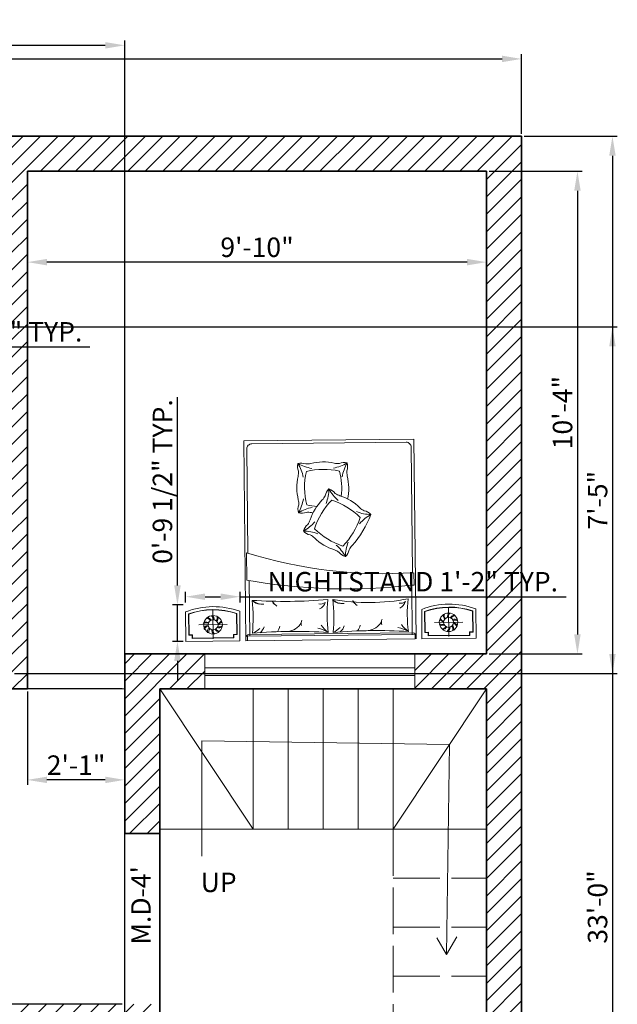
# Model space of a CAD drawing. Units: inches. Extents: x -33 to 381, y -443 to 47.
# Tile 5 of 5: x 228 to 381, y -210 to 43. Entities that reach past the tile are written whole.
import ezdxf

# ---------------------------------------------------------------- set-up
doc = ezdxf.new("R2010")
doc.units = ezdxf.units.IN
doc.linetypes.add('ACAD_ISO02W100', pattern=[15, 12, -3])
for name, color, linetype, lineweight in [('A-ANNO-DIMS', 2, 'Continuous', 18), ('A-ANNO-SYMB', 7, 'Continuous', 18), ('A-ANNO-TEXT', 7, 'Continuous', 18), ('A-DOOR', 4, 'Continuous', 18), ('A-FLOR-STRS', 7, 'Continuous', 18), ('A-FLOR-STRS-OVHD', 8, 'ACAD_ISO02W100', 13), ('A-GLAZ', 4, 'Continuous', 18), ('A-WALL', 7, 'Continuous', 35), ('A-WALL-PATT', 251, 'Continuous', 13), ('furn', 8, 'Continuous', 13)]:
    doc.layers.add(name, color=color, linetype=linetype, lineweight=lineweight)
doc.styles.get("Standard").update_dxf_attribs({"font": 'arial.ttf'})
doc.dimstyles.new('ISO-25', dxfattribs={"dimtxt": 5, "dimasz": 5, "dimexe": 1.25, "dimexo": 0.625, "dimtad": 1, "dimlunit": 3, "dimtxsty": 'Standard', "dimcen": 2.5, "dimadec": 0, "dimazin": 0, "dimtfac": 1, "dimtmove": 0, "dimatfit": 3, "dimfxl": 1, "dimarcsym": 0})

# ---------------------------------------------------------------- blocks, each defined once
blk = doc.blocks.new('*D8')
at = {"layer": 'A-ANNO-DIMS', "color": 0, "lineweight": -2, "transparency": 16777216}
for p, q in [((-3.46, 13.8), (-3.46, 34.29)), ((1.54, 33.04), (351.54, 33.04)), ((356.54, 13.8), (356.54, 34.29))]:
    blk.add_line(p, q, dxfattribs=at)
at = {"layer": 'A-ANNO-DIMS', "color": 0, "transparency": 16777216}
for points in [[(1.54, 33.87), (1.54, 32.21), (-3.46, 33.04)], [(351.54, 33.87), (351.54, 32.21), (356.54, 33.04)]]:
    blk.add_solid(points, dxfattribs=at)
at = {"layer": 'Defpoints', "color": 0, "transparency": 16777216}
for p in [(356.54, 33.04), (-3.46, 13.18), (356.54, 13.18)]:
    blk.add_point(p, dxfattribs=at)
at = {"layer": 'A-ANNO-DIMS', "color": 0, "transparency": 16777216, "insert": (176.54, 36.22), "char_height": 5, "attachment_point": 5}
blk.add_mtext("30'", dxfattribs=at)
blk = doc.blocks.new('NIGHTSTAND-COMPACT')
blk.add_lwpolyline([(0, 7.58), (0.08, 0), (13.98, 0.14), (13.9, 7.73, 0.181818)], format="xyb", close=True)
for points in [[(13.21, 1.73), (13.15, 7.19, 0.167087), (0.76, 7.06), (0.82, 1.6)], [(13.13, 1.73), (13.08, 7.14, 0.165559), (0.84, 7.01), (0.9, 1.6)]]:
    blk.add_lwpolyline(points, format="xyb")
for points in [[(1.74, 0.78), (1.73, 1.69), (0.82, 1.68)], [(1.66, 0.77), (1.66, 1.61), (0.82, 1.6)], [(1.66, 0.85), (12.38, 0.96)], [(1.66, 0.77), (12.38, 0.89)], [(12.31, 0.89), (12.3, 1.8), (13.21, 1.81)], [(12.38, 0.89), (12.37, 1.72), (13.21, 1.73)]]:
    blk.add_lwpolyline(points)
blk = doc.blocks.new('WINDOW-54IN')
for p, q in [((0, 5.5), (54, 5.5)), ((0, 3.5), (54, 3.5))]:
    blk.add_line(p, q)
blk.add_lwpolyline([(0, 9), (54, 9), (54, 0), (0, 0)], close=True)
blk = doc.blocks.new('*D25')
at = {"layer": 'A-ANNO-DIMS', "color": 0, "lineweight": -2, "transparency": 16777216}
for p, q in [((270.19, -106.59), (270.19, -103.87)), ((275.19, -105.12), (279.17, -105.12)), ((284.17, -106.59), (284.17, -103.87)), ((284.17, -105.12), (368, -105.12))]:
    blk.add_line(p, q, dxfattribs=at)
at = {"layer": 'A-ANNO-DIMS', "color": 0, "transparency": 16777216}
for points in [[(275.19, -104.29), (275.19, -105.95), (270.19, -105.12)], [(279.17, -104.29), (279.17, -105.95), (284.17, -105.12)]]:
    blk.add_solid(points, dxfattribs=at)
at = {"layer": 'Defpoints', "color": 0, "transparency": 16777216}
for p in [(284.17, -105.12), (270.19, -107.22), (284.17, -107.22)]:
    blk.add_point(p, dxfattribs=at)
at = {"layer": 'A-ANNO-DIMS', "color": 0, "transparency": 16777216, "insert": (328.58, -101.91), "char_height": 5, "attachment_point": 5}
blk.add_mtext('NIGHTSTAND 1\'-2" TYP.', dxfattribs=at)
blk = doc.blocks.new('*D26')
at = {"layer": 'A-ANNO-DIMS', "color": 0, "lineweight": -2, "transparency": 16777216}
for p, q in [((268.09, -102.22), (268.09, -53.84)), ((269.56, -107.22), (266.84, -107.22)), ((268.09, -116.59), (268.09, -107.22)), ((269.56, -116.59), (266.84, -116.59)), ((268.09, -121.59), (268.09, -126.59))]:
    blk.add_line(p, q, dxfattribs=at)
at = {"layer": 'A-ANNO-DIMS', "color": 0, "transparency": 16777216}
for points in [[(267.25, -102.22), (268.92, -102.22), (268.09, -107.22)], [(267.25, -121.59), (268.92, -121.59), (268.09, -116.59)]]:
    blk.add_solid(points, dxfattribs=at)
at = {"layer": 'Defpoints', "color": 0, "transparency": 16777216}
for p in [(268.09, -107.22), (270.19, -107.22), (270.19, -116.59)]:
    blk.add_point(p, dxfattribs=at)
at = {"layer": 'A-ANNO-DIMS', "color": 0, "transparency": 16777216, "insert": (264.88, -75.53), "char_height": 5, "attachment_point": 5, "rotation": 90}
blk.add_mtext('0\'-9 1/2" TYP.', dxfattribs=at)
blk = doc.blocks.new('*D29')
at = {"layer": 'A-ANNO-DIMS', "color": 0, "lineweight": -2, "transparency": 16777216}
for p, q in [((138.2, -36.45), (138.2, -42.17)), ((172.2, -36.45), (172.2, -42.17)), ((143.2, -40.92), (167.2, -40.92)), ((172.2, -40.92), (245.61, -40.92))]:
    blk.add_line(p, q, dxfattribs=at)
at = {"layer": 'A-ANNO-DIMS', "color": 0, "transparency": 16777216}
for points in [[(143.2, -40.09), (143.2, -41.75), (138.2, -40.92)], [(167.2, -40.09), (167.2, -41.75), (172.2, -40.92)]]:
    blk.add_solid(points, dxfattribs=at)
at = {"layer": 'Defpoints', "color": 0, "transparency": 16777216}
for p in [(138.2, -35.82), (172.2, -35.82), (172.2, -40.92)]:
    blk.add_point(p, dxfattribs=at)
at = {"layer": 'A-ANNO-DIMS', "color": 0, "transparency": 16777216, "insert": (211.4, -37.71), "char_height": 5, "attachment_point": 5}
blk.add_mtext('WINDOW 2\'-10" TYP.', dxfattribs=at)
blk = doc.blocks.new('*D39')
at = {"layer": 'A-ANNO-DIMS', "color": 0, "lineweight": -2, "transparency": 16777216}
for p, q in [((357.17, 13.18), (381.14, 13.18)), ((379.89, 8.18), (379.89, -377.82)), ((357.17, -382.82), (381.14, -382.82))]:
    blk.add_line(p, q, dxfattribs=at)
at = {"layer": 'A-ANNO-DIMS', "color": 0, "transparency": 16777216}
for points in [[(379.06, 8.18), (380.72, 8.18), (379.89, 13.18)], [(379.06, -377.82), (380.72, -377.82), (379.89, -382.82)]]:
    blk.add_solid(points, dxfattribs=at)
at = {"layer": 'Defpoints', "color": 0, "transparency": 16777216}
for p in [(356.54, 13.18), (356.54, -382.82), (379.89, -382.82)]:
    blk.add_point(p, dxfattribs=at)
at = {"layer": 'A-ANNO-DIMS', "color": 0, "transparency": 16777216, "insert": (376.71, -184.82), "char_height": 5, "attachment_point": 5, "rotation": 90}
blk.add_mtext('33\'-0"', dxfattribs=at)
blk = doc.blocks.new('*D42')
at = {"layer": 'A-ANNO-DIMS', "color": 0, "lineweight": -2, "transparency": 16777216}
for p, q in [((229.54, 3.55), (229.54, -20.42)), ((347.54, 3.55), (347.54, -20.42)), ((342.54, -19.17), (234.54, -19.17))]:
    blk.add_line(p, q, dxfattribs=at)
at = {"layer": 'A-ANNO-DIMS', "color": 0, "transparency": 16777216}
for points in [[(234.54, -18.34), (234.54, -20), (229.54, -19.17)], [(342.54, -18.34), (342.54, -20), (347.54, -19.17)]]:
    blk.add_solid(points, dxfattribs=at)
at = {"layer": 'Defpoints', "color": 0, "transparency": 16777216}
for p in [(229.54, 4.18), (347.54, 4.18), (229.54, -19.17)]:
    blk.add_point(p, dxfattribs=at)
at = {"layer": 'A-ANNO-DIMS', "color": 0, "transparency": 16777216, "insert": (288.54, -15.99), "char_height": 5, "attachment_point": 5}
blk.add_mtext('9\'-10"', dxfattribs=at)
blk = doc.blocks.new('*D47')
at = {"layer": 'A-ANNO-DIMS', "color": 0, "lineweight": -2, "transparency": 16777216}
for p, q in [((129.54, -218.2), (129.54, 37.78)), ((134.54, 36.53), (249.54, 36.53)), ((254.54, -218.2), (254.54, 37.78))]:
    blk.add_line(p, q, dxfattribs=at)
at = {"layer": 'A-ANNO-DIMS', "color": 0, "transparency": 16777216}
for points in [[(134.54, 37.36), (134.54, 35.7), (129.54, 36.53)], [(249.54, 37.36), (249.54, 35.7), (254.54, 36.53)]]:
    blk.add_solid(points, dxfattribs=at)
at = {"layer": 'Defpoints', "color": 0, "transparency": 16777216}
for p in [(254.54, 36.53), (129.54, -218.82), (254.54, -218.82)]:
    blk.add_point(p, dxfattribs=at)
at = {"layer": 'A-ANNO-DIMS', "color": 0, "transparency": 16777216, "insert": (192.04, 39.71), "char_height": 5, "attachment_point": 5}
blk.add_mtext('10\'-5"', dxfattribs=at)
blk = doc.blocks.new('*D49')
at = {"layer": 'A-ANNO-DIMS', "color": 0, "lineweight": -2, "transparency": 16777216}
for p, q in [((348.17, 4.18), (372.14, 4.18)), ((370.89, -0.82), (370.89, -114.82)), ((348.17, -119.82), (372.14, -119.82))]:
    blk.add_line(p, q, dxfattribs=at)
at = {"layer": 'A-ANNO-DIMS', "color": 0, "transparency": 16777216}
for points in [[(370.06, -0.82), (371.72, -0.82), (370.89, 4.18)], [(370.06, -114.82), (371.72, -114.82), (370.89, -119.82)]]:
    blk.add_solid(points, dxfattribs=at)
at = {"layer": 'Defpoints', "color": 0, "transparency": 16777216}
for p in [(347.54, 4.18), (347.54, -119.82), (370.89, -119.82)]:
    blk.add_point(p, dxfattribs=at)
at = {"layer": 'A-ANNO-DIMS', "color": 0, "transparency": 16777216, "insert": (367.71, -57.82), "char_height": 5, "attachment_point": 5, "rotation": 90}
blk.add_mtext('10\'-4"', dxfattribs=at)
blk = doc.blocks.new('*D54')
at = {"layer": 'A-ANNO-DIMS', "color": 0, "lineweight": -2, "transparency": 16777216}
for p, q in [((226.17, -35.82), (381.14, -35.82)), ((379.89, -40.82), (379.89, -119.82)), ((226.17, -124.82), (381.14, -124.82))]:
    blk.add_line(p, q, dxfattribs=at)
at = {"layer": 'A-ANNO-DIMS', "color": 0, "transparency": 16777216}
for points in [[(379.06, -40.82), (380.72, -40.82), (379.89, -35.82)], [(379.06, -119.82), (380.72, -119.82), (379.89, -124.82)]]:
    blk.add_solid(points, dxfattribs=at)
at = {"layer": 'Defpoints', "color": 0, "transparency": 16777216}
for p in [(225.54, -35.82), (225.54, -124.82), (379.89, -124.82)]:
    blk.add_point(p, dxfattribs=at)
at = {"layer": 'A-ANNO-DIMS', "color": 0, "transparency": 16777216, "insert": (376.72, -80.32), "char_height": 5, "attachment_point": 5, "rotation": 90}
blk.add_mtext('7\'-5"', dxfattribs=at)
blk = doc.blocks.new('*D57')
at = {"layer": 'A-ANNO-DIMS', "color": 0, "lineweight": -2, "transparency": 16777216}
for p, q in [((253.92, -128.82), (-28.06, -128.82)), ((-26.81, -133.82), (-26.81, -204.82)), ((253.92, -209.82), (-28.06, -209.82))]:
    blk.add_line(p, q, dxfattribs=at)
at = {"layer": 'A-ANNO-DIMS', "color": 0, "transparency": 16777216}
for points in [[(-27.64, -133.82), (-25.98, -133.82), (-26.81, -128.82)], [(-27.64, -204.82), (-25.98, -204.82), (-26.81, -209.82)]]:
    blk.add_solid(points, dxfattribs=at)
at = {"layer": 'Defpoints', "color": 0, "transparency": 16777216}
for p in [(254.54, -128.82), (-26.81, -209.82), (254.54, -209.82)]:
    blk.add_point(p, dxfattribs=at)
at = {"layer": 'A-ANNO-DIMS', "color": 0, "transparency": 16777216, "insert": (-29.99, -169.32), "char_height": 5, "attachment_point": 5, "rotation": 90}
blk.add_mtext('6\'-9"', dxfattribs=at)
blk = doc.blocks.new('*D66')
at = {"layer": 'A-ANNO-DIMS', "color": 0, "lineweight": -2, "transparency": 16777216}
for p, q in [((229.54, -129.45), (229.54, -153.42)), ((254.54, -129.45), (254.54, -153.42)), ((249.54, -152.17), (234.54, -152.17))]:
    blk.add_line(p, q, dxfattribs=at)
at = {"layer": 'A-ANNO-DIMS', "color": 0, "transparency": 16777216}
for points in [[(234.54, -151.34), (234.54, -153), (229.54, -152.17)], [(249.54, -151.34), (249.54, -153), (254.54, -152.17)]]:
    blk.add_solid(points, dxfattribs=at)
at = {"layer": 'Defpoints', "color": 0, "transparency": 16777216}
for p in [(229.54, -128.82), (254.54, -128.82), (229.54, -152.17)]:
    blk.add_point(p, dxfattribs=at)
at = {"layer": 'A-ANNO-DIMS', "color": 0, "transparency": 16777216, "insert": (242.04, -149.03), "char_height": 5, "attachment_point": 5}
blk.add_mtext('2\'-1"', dxfattribs=at)

msp = doc.modelspace()

# ---------------------------------------------------------------- hatches: boundary and pattern name
at = {"layer": 'A-WALL-PATT'}
h = msp.add_hatch(dxfattribs=at)
h.set_pattern_fill('ANSI31', color=256)
h.set_pattern_definition([(45, (-607.8963, -64.2963), (-2.245064, 2.245064), [])])
h.paths.add_polyline_path([(356.541, 13.18), (-3.459, 13.18), (-3.459, -346.82), (-3.459, -382.82), (254.541, -382.82), (254.541, -378.82), (5.541, -378.82), (5.541, -346.82), (36.25, -346.82), (36.25, -337.82), (5.541, -337.82), (5.541, 4.18), (125.541, 4.18), (125.541, -123.82), (129.541, -123.82), (129.541, -76.862), (147.541, -76.862), (147.541, -72.862), (129.541, -72.862), (129.541, 4.18), (225.541, 4.18), (225.541, -124.82), (181.541, -124.82), (181.541, -120.82), (177.541, -120.82), (177.541, -128.82), (229.541, -128.82), (229.541, 4.18), (347.541, 4.18), (347.541, -119.82), (329.098, -119.82), (329.098, -128.82), (347.541, -128.82), (347.541, -373.82), (343.541, -373.82), (343.541, -382.82), (356.541, -382.82), (356.541, -346.82)])
h.paths.add_polyline_path([(181.541, -35.82), (188.17, -35.82), (188.17, -31.82), (172.2, -31.82), (172.2, -35.82), (177.541, -35.82), (177.541, -90.82), (181.541, -90.82)], flags=17)
h.paths.add_polyline_path([(225.541, -31.82), (222.17, -31.82), (222.17, -35.82), (225.541, -35.82)], flags=17)
h.paths.add_polyline_path([(138.2, -31.82), (129.541, -31.82), (129.541, -35.82), (138.2, -35.82)], flags=17)
h.paths.add_polyline_path([(89.541, -167.82), (85.541, -167.82), (85.541, -209.82), (5.541, -209.82), (5.541, -218.82), (90.906, -218.82), (90.906, -209.82), (89.541, -209.82)], flags=17)
h.paths.add_polyline_path([(165.541, -209.82), (125.541, -209.82), (121.541, -209.82), (121.541, -218.82), (125.541, -218.82), (125.541, -310.82), (160.374, -310.82), (160.374, -301.82), (129.541, -301.82), (129.541, -218.82), (165.541, -218.82)], flags=17)
h.paths.add_polyline_path([(263.541, -209.82), (254.541, -209.82), (201.541, -209.82), (201.541, -218.82), (254.541, -218.82), (254.541, -301.82), (214.374, -301.82), (214.374, -310.82), (254.541, -310.82), (263.541, -310.82)], flags=17)
h.paths.add_polyline_path([(263.541, -128.82), (275.098, -128.82), (275.098, -119.82), (254.541, -119.82), (254.541, -128.82), (254.541, -165.974), (263.541, -165.974)], flags=17)
h.paths.add_polyline_path([(263.541, -373.82), (254.541, -373.82), (254.541, -382.82), (263.541, -382.82)], flags=17)

# ---------------------------------------------------------------- linework, layer by layer
at = {"layer": 'A-ANNO-SYMB'}
for p, q in [((274.352, -171.741), (274.352, -142.156)), ((274.352, -142.156), (338.017, -143.106)), ((338.017, -143.106), (337.212, -197.035)), ((337.212, -197.035), (334.745, -192.763)), ((337.212, -197.035), (339.861, -192.446))]:
    msp.add_line(p, q, dxfattribs=at)
at = {"layer": 'A-DOOR'}
msp.add_line((229.541, -128.82), (254.541, -128.82), dxfattribs=at)
at = {"layer": 'A-FLOR-STRS'}
for p, q in [((287.541, -164.82), (263.541, -128.82)), ((287.541, -128.82), (287.541, -164.82)), ((296.541, -128.82), (296.541, -164.82)), ((305.541, -128.82), (305.541, -164.82)), ((314.541, -128.82), (314.541, -164.82)), ((323.541, -128.82), (323.541, -164.82)), ((323.541, -128.82), (323.541, -164.82)), ((323.541, -164.82), (347.541, -128.82)), ((347.541, -164.82), (263.541, -164.82))]:
    msp.add_line(p, q, dxfattribs=at)
at = {"layer": 'A-FLOR-STRS-OVHD'}
for p, q in [((323.541, -164.82), (323.541, -241.188)), ((323.541, -164.82), (347.541, -164.82)), ((323.541, -177.409), (347.541, -177.409)), ((323.541, -189.998), (347.541, -189.998)), ((323.541, -202.587), (347.541, -202.587))]:
    msp.add_line(p, q, dxfattribs=at)
at = {"layer": 'A-WALL'}
for p, q in [((-3.459, 13.18), (356.541, 13.18)), ((356.541, 13.18), (356.541, -346.82)), ((229.541, 4.18), (347.541, 4.18)), ((229.541, -128.82), (229.541, 4.18)), ((347.541, 4.18), (347.541, -119.82)), ((254.541, -119.82), (347.541, -119.82)), ((254.541, -128.82), (254.541, -119.82)), ((229.541, -128.82), (177.541, -128.82)), ((254.541, -128.82), (254.541, -165.974)), ((263.541, -128.82), (263.541, -310.82)), ((263.541, -128.82), (347.541, -128.82)), ((347.541, -128.82), (347.541, -373.82)), ((263.541, -165.974), (254.541, -165.974))]:
    msp.add_line(p, q, dxfattribs=at)
at = {"layer": 'furn'}
for p, q in [((286.673, -115.23), (286.524, -100.96)), ((328.431, -114.794), (328.299, -102.167)), ((277.206, -108.677), (277.283, -115.967)), ((337.733, -108.045), (337.809, -115.336)), ((273.599, -112.36), (280.89, -112.284)), ((341.417, -111.653), (334.126, -111.729)), ((328.643, -114.414), (286.427, -114.855))]:
    msp.add_line(p, q, dxfattribs=at)
for points in [[(329.418, -115.968), (328.882, -64.651), (285.149, -65.108), (285.685, -116.425)], [(286.093, -116.421), (286.081, -115.236), (329.153, -114.786), (329.165, -115.971), (285.685, -116.425)]]:
    msp.add_lwpolyline(points, dxfattribs=at)
for points in [[(328.482, -98.97), (328.145, -66.682, 0.4142136), (326.868, -65.431), (287.179, -65.845, 0.4142136), (285.929, -67.123), (286.209, -93.954)], [(308.157, -72.087, 0.0912961), (311.697, -70.755, 0.0912961), (310.428, -74.318, 0.0912961)], [(299.058, -70.887, 0.1594612), (299.166, -72.877, -0.0762829), (299.092, -74.207, 0.1150751), (299.155, -80.207, -0.0762829), (299.256, -81.535, 0.1594612), (299.19, -83.527)], [(300.401, -74.423, 0.0912961), (299.058, -70.887, 0.0912961), (302.625, -72.145)], [(309.724, -72.84, 0.1110065), (301.221, -72.937, 0.1195491), (301.311, -81.544, 0.0332124), (303.93, -81.914)], [(307.028, -77.431, 0.1594612), (306.068, -79.177, -0.0762829), (305.302, -80.267, 0.1150751), (302.182, -85.393, -0.0762829), (301.566, -86.573, 0.1594612), (300.456, -88.228)], [(306.299, -81.142, 0.0912961), (307.028, -77.431, 0.0912961), (309.391, -80.385)], [(302.73, -82.195, 0.0912961), (299.19, -83.527, 0.0912961), (300.459, -79.964, 0.0912961)], [(315.049, -84.73, 0.1110065), (307.781, -80.315, 0.1195491), (303.305, -87.668, 0.1078134), (310.551, -92.102)], [(314.117, -83.262, 0.0912961), (317.826, -84.003, 0.0912961), (314.864, -86.356, 0.0912961)], [(304.165, -88.97, 0.0912961), (300.456, -88.228, 0.0912961), (303.418, -85.876, 0.0912961)], [(310.59, -92.093, 0.1218652), (315.048, -84.73, 0.1218652)], [(311.983, -91.089, 0.0912961), (311.253, -94.801, 0.0912961), (308.891, -91.847, 0.0912961)]]:
    msp.add_lwpolyline(points, format="xyb", dxfattribs=at)
for points in [[(328.892, -102.16), (328.299, -102.167, -0.0729439), (285.93, -100.844), (285.857, -93.833, 0.0925678), (328.858, -98.944)], [(306.756, -105.846, 0.0585956), (306.844, -114.294, 0.0366479), (287.36, -114.497, 0.052163), (287.272, -106.049, 0.0369674)], [(327.371, -105.631, 0.0585956), (327.459, -114.078, 0.0368889), (308.102, -114.281, 0.052163), (308.014, -105.833, 0.0931113)]]:
    msp.add_lwpolyline(points, format="xyb", close=True, dxfattribs=at)
for centre, radius in [((277.244, -112.322), 2.382), ((277.244, -112.322), 1.29), ((337.771, -111.691), 2.382), ((337.771, -111.691), 1.29)]:
    msp.add_circle(centre, radius, dxfattribs=at)
for centre, radius, start, end in [((299.875, -74.461), 3.666, 71.30055, 102.88227), ((305.554, -83.704), 13.209, 77.65579, 103.91358), ((309.268, -66.503), 4.389, 258.29699, 275.74594), ((310.878, -73.853), 3.204, 75.17738, 111.41808), ((308.62, -71.65), 3.204, 339.96484, 16.20554), ((301.37, -66.611), 4.389, 265.82343, 283.27238), ((292.385, -77.366), 17.92, 353.79379, 14.62661), ((316.007, -73.081), 4.389, 175.63697, 193.08592), ((298.9, -77.209), 13.209, 347.46934, 13.72712), ((305.832, -80.897), 3.666, 39.37364, 70.95536), ((311.252, -75.025), 4.389, 233.89652, 251.34547), ((305.764, -91.745), 13.209, 45.72888, 71.98666), ((300.104, -80.713), 2.959, 251.99778, 292.17564), ((301.66, -87.82), 4.389, 78.29699, 95.74594), ((318.013, -79.11), 4.389, 226.37008, 243.81903), ((315.492, -86.199), 3.204, 43.25047, 79.49116), ((305.375, -70.619), 13.209, 257.65579, 259.30153), ((292.093, -73.796), 27.683, 318.98002, 338.36262), ((302.721, -86.324), 2.959, 220.07087, 260.24873), ((300.283, -93.179), 4.389, 46.37008, 63.81903), ((312.532, -80.544), 13.209, 225.72888, 251.98666), ((307.043, -97.264), 4.389, 53.89652, 71.34547), ((309.066, -92.46), 3.204, 313.06401, 349.30471), ((316.147, -95.004), 4.389, 136.18362, 153.63258), ((312.07, -91.819), 3.092, 217.89195, 254.69556), ((289.209, -104.817), 2.189, 214.2331, 271.44382), ((289.842, -103.605), 3.455, 225.00427, 277.43246), ((310.457, -103.39), 3.455, 225.00427, 277.43246), ((309.824, -104.601), 2.189, 214.2331, 271.44382), ((313.871, -106.13), 0.709, 174.35251, 257.81689), ((321.613, -99.814), 10.554, 216.80675, 225.68314), ((293.256, -106.345), 0.709, 174.35251, 257.81689), ((300.998, -100.029), 10.554, 216.80675, 225.68314), ((304.878, -105.083), 1.921, 257.08052, 309.1545), ((303.426, -105.686), 2.809, 294.88983, 341.58783), ((325.494, -104.868), 1.921, 257.08052, 309.1545), ((324.041, -105.471), 2.809, 294.88983, 341.58783), ((275.556, -111.857), 1.167, 32.06021, 92.29806), ((275.479, -111.99), 1.53, 34.10848, 80.4282), ((276.151, -110.954), 1.167, 356.06021, 56.29806), ((276.012, -111.016), 1.53, 358.10848, 44.4282), ((277.164, -110.572), 1.167, 320.06021, 20.29806), ((277.015, -110.541), 1.53, 322.10848, 8.4282), ((278.208, -110.859), 1.167, 284.06021, 344.29806), ((301.987, -111.942), 2.1, 156.49097, 196.71742), ((322.602, -111.727), 2.1, 156.49097, 196.71742), ((336.877, -110.133), 1.53, 208.76826, 255.08798), ((336.777, -110.249), 1.167, 196.8984, 257.13625), ((337.963, -109.905), 1.53, 172.76826, 219.08798), ((337.815, -109.94), 1.167, 160.8984, 221.13625), ((338.976, -110.359), 1.53, 136.76826, 183.08798), ((338.836, -110.3), 1.167, 124.8984, 185.13625), ((339.529, -111.322), 1.53, 100.76826, 147.08798), ((339.45, -111.191), 1.167, 88.8984, 149.13625), ((339.41, -112.426), 1.53, 64.76826, 111.08798), ((339.423, -112.273), 1.167, 52.8984, 113.13625), ((275.432, -113.006), 1.167, 68.06021, 128.29806), ((275.448, -113.158), 1.53, 70.10848, 116.4282), ((276.21, -113.966), 1.53, 106.10848, 152.4282), ((276.108, -113.852), 1.167, 104.06021, 164.29806), ((277.301, -114.171), 1.53, 142.10848, 188.4282), ((277.324, -114.072), 1.167, 140.06021, 200.29806), ((278.477, -113.629), 1.53, 178.10848, 224.4282), ((278.338, -113.691), 1.167, 176.06021, 236.29806), ((279.01, -112.654), 1.53, 214.10848, 260.4282), ((278.933, -112.787), 1.167, 212.06021, 272.29806), ((278.868, -111.553), 1.53, 250.10848, 296.4282), ((278.884, -111.705), 1.167, 248.06021, 308.29806), ((278.106, -110.746), 1.53, 286.10848, 332.4282), ((284.77, -108.733), 6.371, 295.24388, 314.75671), ((287.006, -111.69), 3.536, 311.13366, 340.95404), ((291.168, -112.112), 3.286, 322.41563, 350.49689), ((295.878, -109.398), 4.686, 277.28316, 328.91643), ((302.425, -121.403), 8.371, 58.13614, 78.12153), ((313.096, -106.327), 10.126, 217.09176, 231.87742), ((305.385, -108.518), 6.371, 295.24388, 314.75671), ((307.622, -111.474), 3.536, 311.13366, 340.95404), ((311.783, -111.897), 3.286, 322.41563, 350.49689), ((316.493, -109.183), 4.686, 277.28316, 328.91643), ((323.04, -121.188), 8.371, 58.13614, 78.12153), ((333.711, -106.112), 10.126, 217.09176, 231.87742), ((336.119, -111.108), 1.167, 232.8984, 293.13625), ((336.132, -110.956), 1.53, 244.76826, 291.08798), ((336.092, -112.191), 1.167, 268.8984, 329.13625), ((336.013, -112.06), 1.53, 280.76826, 327.08798), ((336.707, -113.082), 1.167, 304.8984, 5.13625), ((336.566, -113.023), 1.53, 316.76826, 3.08798), ((337.728, -113.442), 1.167, 340.8984, 41.13625), ((337.579, -113.477), 1.53, 352.76826, 39.08798), ((338.765, -113.133), 1.167, 16.8984, 77.13625), ((338.665, -113.249), 1.53, 28.76826, 75.08798), ((286.435, -115.613), 0.758, 90.59823, 180.59823), ((328.651, -115.172), 0.758, 0.59823, 90.59823)]:
    msp.add_arc(centre, radius, start, end, dxfattribs=at)

# ---------------------------------------------------------------- block references
at = {"layer": 'A-GLAZ'}
msp.add_blockref('WINDOW-54IN', (275.097, -128.863), dxfattribs=at)
at = {"layer": 'furn'}
msp.add_blockref('NIGHTSTAND-COMPACT', (270.185, -116.585), dxfattribs=at)
at = {"layer": 'furn', "extrusion": (0, 0, -1), "zscale": -1, "rotation": 358.8035477638503}
msp.add_blockref('NIGHTSTAND-COMPACT', (-344.918, -115.802), dxfattribs=at)

# ---------------------------------------------------------------- texts
at = {"layer": 'A-ANNO-TEXT', "insert": (256.198, -194.485), "char_height": 5, "attachment_point": 1, "rotation": 90}
msp.add_mtext_dynamic_manual_height_columns("M.D-4'", width=18.76148, gutter_width=12.5, heights=[0], dxfattribs=at)
at = {"layer": 'A-ANNO-TEXT', "insert": (274.061, -175.99), "char_height": 5, "attachment_point": 1}
msp.add_mtext_dynamic_manual_height_columns('UP', width=14.62948, gutter_width=12.5, heights=[0], dxfattribs=at)

# ---------------------------------------------------------------- dimensions: what is measured, and where the dimension line sits
at = {"layer": 'A-ANNO-DIMS'}
for base, p1, p2, override, picture, middle in [((254.541, 36.53), (129.541, -218.82), (254.541, -218.82), {"dimdec": 1, "dimlfac": 1, "dimrnd": 0, "dimzin": 1, "dimdsep": 46, "dimlunit": 4, "dimfrac": 2}, '*D47', (192.041, 39.708)), ((356.541, 33.041), (-3.459, 13.18), (356.541, 13.18), {"dimclrd": 0, "dimclre": 0, "dimclrt": 0}, '*D8', (176.541, 36.221))]:
    dim = msp.add_linear_dim(base=base, p1=p1, p2=p2, dimstyle='ISO-25', override=override, dxfattribs=at)
    dim.commit()
    dim.dimension.update_dxf_attribs({"geometry": picture, "text_midpoint": middle})
for base, p1, p2, angle, picture, middle in [((379.891, -382.82), (356.541, 13.18), (356.541, -382.82), 270, '*D39', (376.712, -184.82)), ((229.541, -19.17), (347.541, 4.18), (229.541, 4.18), 180, '*D42', (288.541, -15.992)), ((370.891, -119.82), (347.541, 4.18), (347.541, -119.82), 270, '*D49', (367.713, -57.82)), ((379.891, -124.82), (225.541, -35.82), (225.541, -124.82), 90, '*D54', (376.723, -80.32)), ((-26.809, -209.82), (254.541, -128.82), (254.541, -209.82), 90, '*D57', (-29.987, -169.32)), ((229.541, -152.17), (254.541, -128.82), (229.541, -128.82), 180, '*D66', (242.041, -149.035))]:
    dim = msp.add_linear_dim(base=base, p1=p1, p2=p2, angle=angle, dimstyle='ISO-25', override={"dimdec": 1, "dimlfac": 1, "dimrnd": 0, "dimzin": 1, "dimdsep": 46, "dimlunit": 4, "dimfrac": 2}, dxfattribs=at)
    dim.commit()
    dim.dimension.update_dxf_attribs({"geometry": picture, "text_midpoint": middle})
for base, p1, p2, text, picture, middle in [((172.2, -40.92), (138.2, -35.82), (172.2, -35.82), 'WINDOW <> TYP.', '*D29', (211.403, -37.708)), ((284.168, -105.121), (270.185, -107.218), (284.168, -107.218), 'NIGHTSTAND <> TYP.', '*D25', (328.582, -101.91))]:
    dim = msp.add_linear_dim(base=base, p1=p1, p2=p2, text=text, dimstyle='ISO-25', override={"dimdec": 1, "dimlfac": 1, "dimrnd": 0, "dimzin": 1, "dimdsep": 46, "dimlunit": 4, "dimfrac": 2}, dxfattribs=at)
    dim.commit()
    dim.dimension.update_dxf_attribs({"geometry": picture, "text_midpoint": middle})
dim = msp.add_linear_dim(base=(268.088, -107.218), p1=(270.185, -116.585), p2=(270.185, -107.218), angle=90, text='<> TYP.', dimstyle='ISO-25', override={"dimdec": 1, "dimlfac": 1, "dimrnd": 0, "dimzin": 1, "dimdsep": 46, "dimlunit": 4, "dimfrac": 2}, dxfattribs=at)
dim.commit()
dim.dimension.update_dxf_attribs({"geometry": '*D26', "text_midpoint": (264.878, -75.529)})

doc.saveas('drawing.dxf')
